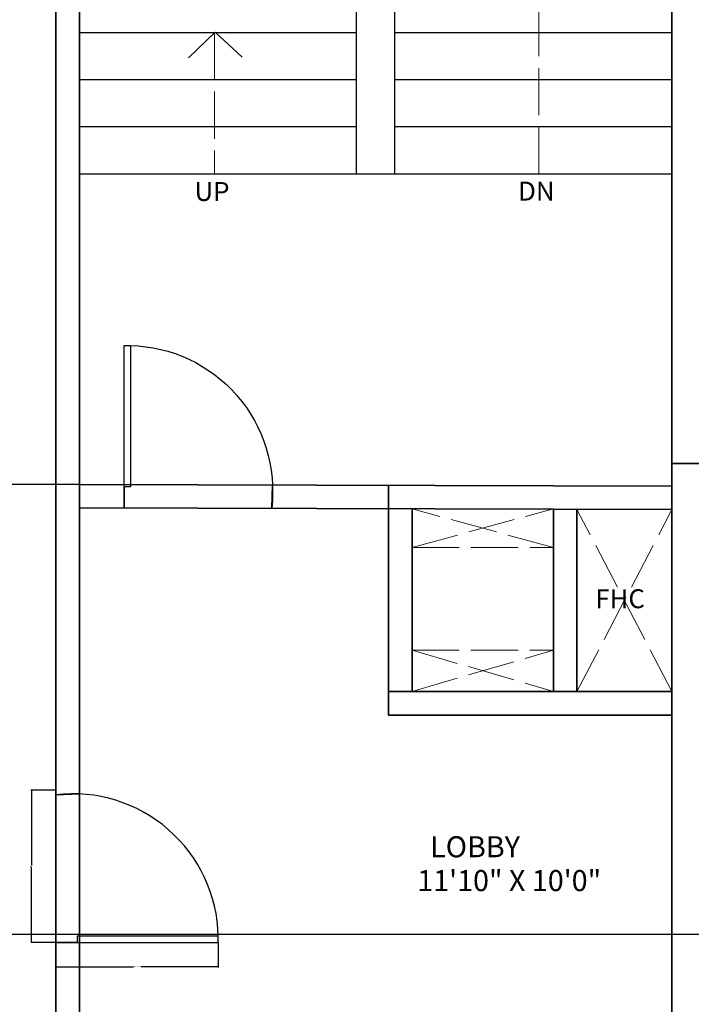
# Model space of a CAD drawing. Units: inches. Extents: x -61 to 1599, y -1316 to 257.
# Tile 183 of 204: x 826 to 998, y -579 to -328. Entities that reach past the tile are written whole.
import ezdxf

# ---------------------------------------------------------------- set-up
doc = ezdxf.new("R2010")
doc.units = ezdxf.units.IN
doc.header["$MEASUREMENT"] = 0
doc.linetypes.add('ACAD_ISO02W100', pattern=[15, 12, -3])
for name, color, linetype, lineweight in [('A-ANNO-DIMS', 2, 'Continuous', 18), ('A-ANNO-SYMB', 1, 'Continuous', 18), ('A-AREA-IDEN', 1, 'Continuous', 18), ('A-FLOR-OPEN-HIDN', 8, 'ACAD_ISO02W100', 13), ('A-FLOR-STRS', 8, 'Continuous', 25), ('A-FLOR-STRS-PATH', 8, 'ACAD_ISO02W100', 13), ('A-WALL-JAMB', 4, 'ACAD_ISO02W100', 25), ('DOORS', 2, 'Continuous', 25), ('WALLS', 4, 'Continuous', 35)]:
    doc.layers.add(name, color=color, linetype=linetype, lineweight=lineweight)
doc.styles.get("Standard").update_dxf_attribs({"font": 'arial.ttf'})
doc.dimstyles.get("Standard").update_dxf_attribs({"dimtxt": 0.18, "dimasz": 0.18, "dimexe": 0.18, "dimexo": 0.0625, "dimgap": 0.09, "dimtad": 0, "dimtih": 1, "dimtoh": 1, "dimdec": 0, "dimzin": 0, "dimdsep": 46, "dimlunit": 3, "dimtxsty": 'Standard', "dimcen": 0.09, "dimadec": 0, "dimazin": 0, "dimtfac": 1, "dimtdec": 0, "dimtofl": 0, "dimtmove": 0, "dimatfit": 3, "dimfxl": 1, "dimtolj": 1, "dimtzin": 0, "dimarcsym": 0})

# ---------------------------------------------------------------- blocks, each defined once
blk = doc.blocks.new('DOOR-SWING-36')
blk.add_line((0, 0), (0, -5.4))
blk.add_lwpolyline([(0, 0), (0, 36), (-1.57, 36), (-1.57, 0)], close=True)
blk.add_arc((-0.74, -1.08), 37.09, 91.2913, 186.6905)
blk = doc.blocks.new('*D622')
at = {"layer": 'A-ANNO-DIMS', "color": 0, "lineweight": -2, "transparency": 16777216}
for p, q in [((835.7, -563.31), (835.7, -569.64)), ((877.1, -563.31), (877.1, -569.64)), ((835.88, -569.46), (855.47, -569.46)), ((876.92, -569.46), (857.34, -569.46))]:
    blk.add_line(p, q, dxfattribs=at)
at = {"layer": 'A-ANNO-DIMS', "color": 0, "transparency": 16777216}
for points in [[(835.88, -569.43), (835.88, -569.49), (835.7, -569.46)], [(876.92, -569.43), (876.92, -569.49), (877.1, -569.46)]]:
    blk.add_solid(points, dxfattribs=at)
at = {"layer": 'DEFPOINTS', "color": 0, "transparency": 16777216}
for p in [(835.7, -563.25), (877.1, -563.25), (877.1, -569.46)]:
    blk.add_point(p, dxfattribs=at)
at = {"layer": 'A-ANNO-DIMS', "color": 0, "transparency": 16777216, "insert": (856.4, -569.46), "char_height": 0.18, "attachment_point": 5}
blk.add_mtext('\\A1;DOOR 41 TYP.', dxfattribs=at)
blk = doc.blocks.new('*D623')
at = {"layer": 'A-ANNO-DIMS', "color": 0, "lineweight": -2, "transparency": 16777216}
for p, q in [((835.64, -524.46), (829.31, -524.46)), ((829.49, -524.64), (829.49, -543.67)), ((829.49, -563.07), (829.49, -544.04)), ((835.64, -563.25), (829.31, -563.25))]:
    blk.add_line(p, q, dxfattribs=at)
at = {"layer": 'A-ANNO-DIMS', "color": 0, "transparency": 16777216}
for points in [[(829.46, -524.64), (829.52, -524.64), (829.49, -524.46)], [(829.46, -563.07), (829.52, -563.07), (829.49, -563.25)]]:
    blk.add_solid(points, dxfattribs=at)
at = {"layer": 'DEFPOINTS', "color": 0, "transparency": 16777216}
for p in [(835.7, -524.46), (829.49, -563.25), (835.7, -563.25)]:
    blk.add_point(p, dxfattribs=at)
at = {"layer": 'A-ANNO-DIMS', "color": 0, "transparency": 16777216, "insert": (829.49, -543.86), "char_height": 0.18, "attachment_point": 5}
blk.add_mtext('\\A1;39 TYP.', dxfattribs=at)
blk = doc.blocks.new('*D697')
at = {"layer": 'A-ANNO-DIMS', "color": 0, "lineweight": -2, "transparency": 16777216}
for p, q in [((644.7, -561.11), (644.7, 257.46)), ((644.88, 257.28), (739.94, 257.28)), ((835.52, 257.28), (740.47, 257.28)), ((835.7, -563.19), (835.7, 257.46))]:
    blk.add_line(p, q, dxfattribs=at)
at = {"layer": 'A-ANNO-DIMS', "color": 0, "transparency": 16777216}
for points in [[(644.88, 257.31), (644.88, 257.25), (644.7, 257.28)], [(835.52, 257.31), (835.52, 257.25), (835.7, 257.28)]]:
    blk.add_solid(points, dxfattribs=at)
at = {"layer": 'DEFPOINTS', "color": 0, "transparency": 16777216}
for p in [(835.7, 257.28), (644.7, -561.17), (835.7, -563.25)]:
    blk.add_point(p, dxfattribs=at)
at = {"layer": 'A-ANNO-DIMS', "color": 0, "transparency": 16777216, "insert": (740.2, 257.28), "char_height": 0.18, "attachment_point": 5}
blk.add_mtext('\\A1;191', dxfattribs=at)
blk = doc.blocks.new('*D698')
at = {"layer": 'A-ANNO-DIMS', "color": 0, "lineweight": -2, "transparency": 16777216}
for p, q in [((644.77, -167.17), (1598.48, -167.17)), ((1598.3, -167.35), (1598.3, -363.99)), ((1598.3, -560.99), (1598.3, -364.35)), ((644.77, -561.17), (1598.48, -561.17))]:
    blk.add_line(p, q, dxfattribs=at)
at = {"layer": 'A-ANNO-DIMS', "color": 0, "transparency": 16777216}
for points in [[(1598.27, -167.35), (1598.33, -167.35), (1598.3, -167.17)], [(1598.27, -560.99), (1598.33, -560.99), (1598.3, -561.17)]]:
    blk.add_solid(points, dxfattribs=at)
at = {"layer": 'DEFPOINTS', "color": 0, "transparency": 16777216}
for p in [(644.7, -167.17), (1598.3, -167.17), (644.7, -561.17)]:
    blk.add_point(p, dxfattribs=at)
at = {"layer": 'A-ANNO-DIMS', "color": 0, "transparency": 16777216, "insert": (1598.3, -364.17), "char_height": 0.18, "attachment_point": 5}
blk.add_mtext('\\A1;394', dxfattribs=at)
blk = doc.blocks.new('*D699')
at = {"layer": 'A-ANNO-DIMS', "color": 0, "lineweight": -2, "transparency": 16777216}
for p, q in [((835.64, -167.17), (-61.08, -167.17)), ((-60.9, -167.35), (-60.9, -306.73)), ((-60.9, -446.47), (-60.9, -307.09)), ((841.64, -446.65), (-61.08, -446.65))]:
    blk.add_line(p, q, dxfattribs=at)
at = {"layer": 'A-ANNO-DIMS', "color": 0, "transparency": 16777216}
for points in [[(-60.93, -167.35), (-60.87, -167.35), (-60.9, -167.17)], [(-60.93, -446.47), (-60.87, -446.47), (-60.9, -446.65)]]:
    blk.add_solid(points, dxfattribs=at)
at = {"layer": 'DEFPOINTS', "color": 0, "transparency": 16777216}
for p in [(835.7, -167.17), (-60.9, -446.65), (841.7, -446.65)]:
    blk.add_point(p, dxfattribs=at)
at = {"layer": 'A-ANNO-DIMS', "color": 0, "transparency": 16777216, "insert": (-60.9, -306.91), "char_height": 0.18, "attachment_point": 5}
blk.add_mtext('\\A1;279.5', dxfattribs=at)

msp = doc.modelspace()

# ---------------------------------------------------------------- linework, layer by layer
at = {"layer": 'A-FLOR-OPEN-HIDN'}
for p, q in [((926.4835, -462.6959), (962.4835, -452.8666)), ((962.4835, -462.6959), (926.4835, -452.8666)), ((992.7028, -499.392), (968.4835, -453.0009)), ((968.4835, -499.392), (992.7028, -453.0686)), ((926.4835, -462.6959), (962.4835, -462.6959)), ((926.4835, -488.8238), (962.4835, -488.8238)), ((926.4835, -488.8238), (962.4835, -499.392)), ((926.4835, -499.392), (962.4835, -488.8238))]:
    msp.add_line(p, q, dxfattribs=at)
at = {"layer": 'A-FLOR-STRS'}
for p, q in [((912.2261, -247.6332), (912.2261, -367.6332)), ((922.0298, -247.6332), (922.0298, -367.6332)), ((912.2261, -331.6332), (841.7028, -331.6332)), ((992.7028, -331.6332), (922.0298, -331.6332)), ((912.2261, -343.6332), (841.7028, -343.6332)), ((992.7028, -343.6332), (922.0298, -343.6332)), ((912.2261, -355.6332), (841.7028, -355.6332)), ((992.7028, -355.6332), (922.0298, -355.6332)), ((992.7028, -367.6332), (841.7028, -367.6332))]:
    msp.add_line(p, q, dxfattribs=at)
at = {"layer": 'A-FLOR-STRS-PATH'}
for p, q in [((958.7606, -367.6332), (958.7606, -212.0484)), ((876.301, -331.4893), (869.5395, -337.9798)), ((876.1511, -331.6332), (876.1511, -367.6332)), ((876.301, -331.4893), (883.183, -337.8518))]:
    msp.add_line(p, q, dxfattribs=at)
at = {"layer": 'A-WALL-JAMB'}
for p, q in [((853.1234, -452.6782), (853.1234, -446.6782)), ((890.6984, -452.6782), (890.9176, -446.7839)), ((835.7028, -525.6774), (841.7028, -525.4628)), ((835.7028, -563.2524), (841.7028, -563.2524))]:
    msp.add_line(p, q, dxfattribs=at)
at = {"layer": 'WALLS'}
for p, q in [((992.7028, 157.6771), (992.7028, -441.3229)), ((835.7028, -61.169), (835.7028, -741.169)), ((841.7028, -61.169), (841.7028, -612.169)), ((992.7028, -61.169), (992.7028, -612.169)), ((992.7028, -441.3229), (1215.7028, -441.3229)), ((992.7196, -447.0686), (841.7028, -446.6462)), ((920.4835, -505.392), (920.4835, -446.8666)), ((992.7028, -453.0686), (841.7028, -452.6463)), ((926.4835, -499.392), (926.4835, -452.8666)), ((962.4835, -499.392), (962.4835, -452.8666)), ((968.4835, -499.392), (968.4835, -452.8666)), ((992.7028, -499.392), (920.4835, -499.392)), ((992.7028, -505.392), (920.4835, -505.392))]:
    msp.add_line(p, q, dxfattribs=at)

# ---------------------------------------------------------------- block references
at = {"layer": 'DOORS', "extrusion": (0, 0, -1), "zscale": -1}
msp.add_blockref('DOOR-SWING-36', (-853.1234, -447.2782), dxfattribs=at)
at = {"layer": 'DOORS', "rotation": 269.9999999999935}
msp.add_blockref('DOOR-SWING-36', (841.1028, -563.2524), dxfattribs=at)

# ---------------------------------------------------------------- texts
at = {"layer": 'A-ANNO-SYMB'}
for s, p in [('UP', (871.0358, -374.4735)), ('DN', (953.4953, -374.3755)), ('FHC', (973.1658, -478.165))]:
    msp.add_text(s, height=4.8321, dxfattribs=at).set_placement(p)
at = {"layer": 'A-AREA-IDEN'}
for s, height, p in [('  LOBBY', 5.35952, (927.8065, -541.5899)), ('11\'10" X 10\'0"', 5.359524, (927.8065, -550.1995))]:
    msp.add_text(s, height=height, dxfattribs=at).set_placement(p)

# ---------------------------------------------------------------- dimensions: what is measured, and where the dimension line sits
at = {"layer": 'A-ANNO-DIMS'}
dim = msp.add_linear_dim(base=(835.7028, 257.2771), p1=(644.7028, -561.169), p2=(835.7028, -563.2524), dimstyle='Standard', override={"dimdec": 0, "dimlfac": 1, "dimrnd": 0, "dimzin": 0, "dimdsep": 46, "dimlunit": 2}, dxfattribs=at)
dim.commit()
dim.dimension.update_dxf_attribs({"geometry": '*D697', "text_midpoint": (740.2028, 257.2771)})
for base, p1, p2, override, picture, middle in [((-60.8972, -446.6462), (835.7028, -167.169), (841.7028, -446.6462), {"dimdec": 1, "dimlfac": 1, "dimrnd": 0, "dimzin": 0, "dimdsep": 46, "dimlunit": 2}, '*D699', (-60.8972, -306.9076)), ((1598.3028, -167.169), (644.7028, -561.169), (644.7028, -167.169), {"dimdec": 0, "dimlfac": 1, "dimrnd": 0, "dimzin": 0, "dimdsep": 46, "dimlunit": 2}, '*D698', (1598.3028, -364.169))]:
    dim = msp.add_linear_dim(base=base, p1=p1, p2=p2, angle=90, dimstyle='Standard', override=override, dxfattribs=at)
    dim.commit()
    dim.dimension.update_dxf_attribs({"geometry": picture, "text_midpoint": middle})
dim = msp.add_linear_dim(base=(829.4928, -563.2524), p1=(835.7028, -524.4606), p2=(835.7028, -563.2524), angle=270, text='<> TYP.', dimstyle='Standard', override={"dimdec": 0, "dimlfac": 1, "dimrnd": 0, "dimzin": 0, "dimdsep": 46, "dimlunit": 2}, dxfattribs=at)
dim.commit()
dim.dimension.update_dxf_attribs({"geometry": '*D623', "text_midpoint": (829.4928, -543.8565)})
dim = msp.add_linear_dim(base=(877.1028, -569.4624), p1=(835.7028, -563.2524), p2=(877.1028, -563.2524), text='DOOR <> TYP.', dimstyle='Standard', override={"dimdec": 0, "dimlfac": 1, "dimrnd": 0, "dimzin": 0, "dimdsep": 46, "dimlunit": 2}, dxfattribs=at)
dim.commit()
dim.dimension.update_dxf_attribs({"geometry": '*D622', "text_midpoint": (856.4028, -569.4624)})

doc.saveas('drawing.dxf')
